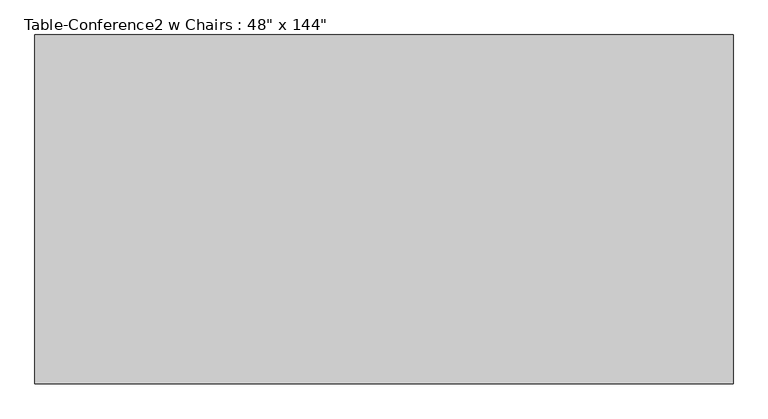
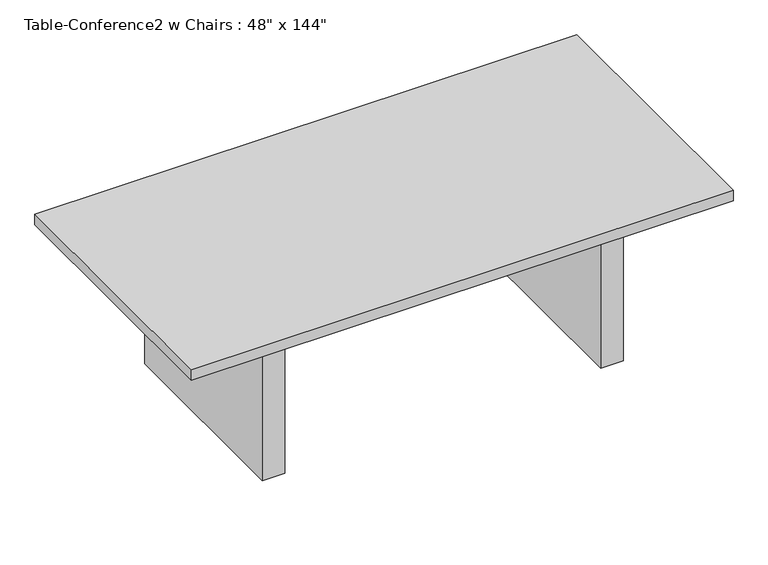
"""IFC4 building model written with IfcOpenShell, lengths in millimetres: furniture geometry."""

from ifc_helpers import new_model, si_unit, frame, origin, origin_with_axes, place, context, project, spatial, polyline, outline, extrude, source, transform, mapped, element, save


def furniture_6f689152(model_context):
    return source(origin(), model_context, "Body", "SweptSolid", [
        extrude(outline(polyline([(1219.2, -609.6), (-1219.2, -609.6), (-1219.2, 609.6), (1219.2, 609.6), (1219.2, -609.6)])), frame((0.0, 0.0, 711.2), z_axis=(0.0, 0.0, 1.0), x_axis=(1.0, 0.0, 0.0)), (0.0, 0.0, 1.0), 50.8),
        extrude(outline(polyline([(-711.2, -457.2), (-812.8, -457.2), (-812.8, 457.2), (-711.2, 457.2), (-711.2, -457.2)])), origin_with_axes(), (0.0, 0.0, 1.0), 711.2),
        extrude(outline(polyline([(812.8, -457.2), (711.2, -457.2), (711.2, 457.2), (812.8, 457.2), (812.8, -457.2)])), origin_with_axes(), (0.0, 0.0, 1.0), 711.2),
        extrude(outline(polyline([(711.2, 457.2), (711.2, 419.1), (-711.2, 419.1), (-711.2, 457.2), (711.2, 457.2)])), frame((0.0, 0.0, 609.6), z_axis=(0.0, 0.0, 1.0), x_axis=(1.0, 0.0, 0.0)), (0.0, 0.0, 1.0), 101.6),
        extrude(outline(polyline([(711.2, -457.2), (-711.2, -457.2), (-711.2, -419.1), (711.2, -419.1), (711.2, -457.2)])), frame((0.0, 0.0, 609.6), z_axis=(0.0, 0.0, 1.0), x_axis=(1.0, 0.0, 0.0)), (0.0, 0.0, 1.0), 101.6),
    ])


if __name__ == "__main__":
    model = new_model("IFC4")
    model_context = context("Model", 3, world=origin())
    ifc_project = project(units=[si_unit("LENGTHUNIT", "METRE", prefix="MILLI")], contexts=[model_context])
    site = spatial("IfcSite", under=ifc_project)
    building = spatial("IfcBuilding", under=site)
    placement = place(None, origin())
    furniture_shape = furniture_6f689152(model_context)
    element("IfcFurniture", 1, ObjectType="Table-Conference2 w Chairs : 48\" x 144\"", at=placement, inside=building, context=model_context, shape_type="MappedRepresentation", body=[
        mapped(furniture_shape, transform((0.0, 0.0, 0.0), x_axis=(1.0, 0.0, 0.0), y_axis=(0.0, 1.0, 0.0), z_axis=(0.0, 0.0, 1.0))),
    ])
    save(model, "model.ifc")

# Revit data of these elements
# Type "Table-Conference2 w Chairs : 48\" x 144\""
#   Assembly Code = "E2020200"
#   Description = "Seating 12-14"
#   Height = 2' - 6"
#   Length = 8' - 0"
#   Width = 4' - 0"
#   Number Of Chairs One Side = 3
#   Number Of Chairs = 8
#   Material = Wood - Cherry
#   Default Elevation = 0
# Element 1 (IfcFurniture, "Table-Conference2 w Chairs : 48\" x 144\"")
#   Materials on its faces: "Wood - Cherry"
# Materials
#   "Wood - Cherry": colour RGB 151 75 0, transparency 0
